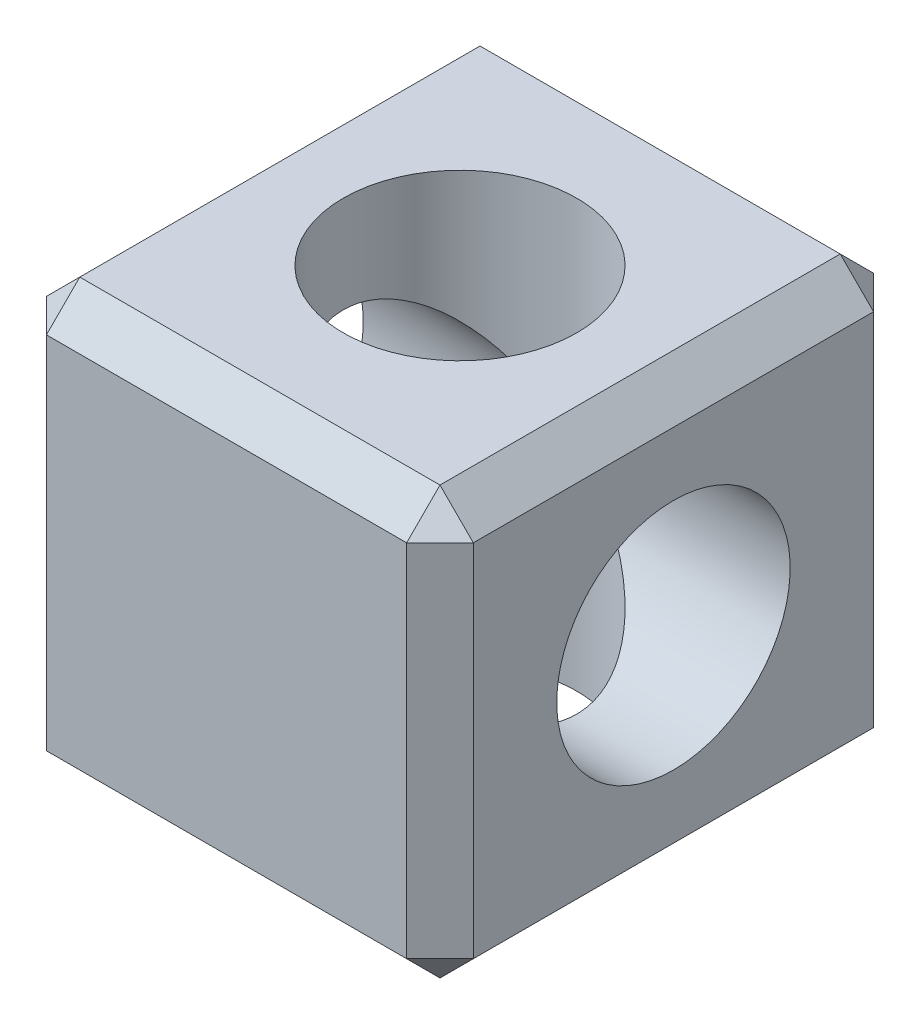
ISO-10303-21;
HEADER;
FILE_DESCRIPTION(('STEP AP214'),'2;1');
FILE_NAME('part.step','',(''),(''),'','','');
FILE_SCHEMA(('AUTOMOTIVE_DESIGN { 1 0 10303 214 1 1 1 1 }'));
ENDSEC;
DATA;
#1=APPLICATION_CONTEXT('core data for automotive mechanical design processes');
#2=APPLICATION_PROTOCOL_DEFINITION('international standard','automotive_design',2000,#1);
#3=PRODUCT_CONTEXT('',#1,'mechanical');
#4=PRODUCT('Part','Part','',(#3));
#5=PRODUCT_RELATED_PRODUCT_CATEGORY('part','',(#4));
#6=PRODUCT_DEFINITION_FORMATION('','',#4);
#7=PRODUCT_DEFINITION_CONTEXT('part definition',#1,'design');
#8=PRODUCT_DEFINITION('design','',#6,#7);
#9=PRODUCT_DEFINITION_SHAPE('','',#8);
#10=(LENGTH_UNIT() NAMED_UNIT(*) SI_UNIT(.MILLI.,.METRE.));
#11=(NAMED_UNIT(*) PLANE_ANGLE_UNIT() SI_UNIT($,.RADIAN.));
#12=(NAMED_UNIT(*) SI_UNIT($,.STERADIAN.) SOLID_ANGLE_UNIT());
#13=UNCERTAINTY_MEASURE_WITH_UNIT(LENGTH_MEASURE(1.E-05),#10,'distance_accuracy_value','');
#14=(GEOMETRIC_REPRESENTATION_CONTEXT(3) GLOBAL_UNCERTAINTY_ASSIGNED_CONTEXT((#13)) GLOBAL_UNIT_ASSIGNED_CONTEXT((#10,
#11,#12)) REPRESENTATION_CONTEXT('',''));
#15=CARTESIAN_POINT('',(0.,0.,0.));
#16=DIRECTION('',(0.,0.,1.));
#17=DIRECTION('',(1.,0.,0.));
#18=AXIS2_PLACEMENT_3D('',#15,#16,#17);
#19=CARTESIAN_POINT('',(0.,-32.,35.));
#20=DIRECTION('',(0.,1.,0.));
#21=DIRECTION('',(-1.,0.,0.));
#22=AXIS2_PLACEMENT_3D('',#19,#20,#21);
#23=CYLINDRICAL_SURFACE('',#22,17.5);
#24=CARTESIAN_POINT('',(0.,32.,35.));
#25=DIRECTION('',(0.,1.,0.));
#26=DIRECTION('',(-1.,0.,0.));
#27=AXIS2_PLACEMENT_3D('',#24,#25,#26);
#28=CIRCLE('',#27,17.5);
#29=CARTESIAN_POINT('',(-17.5,32.,35.));
#30=VERTEX_POINT('',#29);
#31=EDGE_CURVE('E266',#30,#30,#28,.T.);
#32=ORIENTED_EDGE('',*,*,#31,.T.);
#33=EDGE_LOOP('',(#32));
#34=FACE_BOUND('',#33,.T.);
#35=CARTESIAN_POINT('',(0.,0.,35.));
#36=DIRECTION('',(-0.707106781186548,0.707106781186547,0.));
#37=DIRECTION('',(0.707106781186547,0.707106781186548,0.));
#38=AXIS2_PLACEMENT_3D('',#35,#36,#37);
#39=ELLIPSE('',#38,24.7487373415292,17.5);
#40=CARTESIAN_POINT('',(0.,0.,17.5));
#41=VERTEX_POINT('',#40);
#42=CARTESIAN_POINT('',(0.,0.,52.5));
#43=VERTEX_POINT('',#42);
#44=EDGE_CURVE('E145',#41,#43,#39,.F.);
#45=ORIENTED_EDGE('',*,*,#44,.T.);
#46=CARTESIAN_POINT('',(0.,0.,35.));
#47=DIRECTION('',(0.707106781186547,0.707106781186548,0.));
#48=DIRECTION('',(-0.707106781186548,0.707106781186547,0.));
#49=AXIS2_PLACEMENT_3D('',#46,#47,#48);
#50=ELLIPSE('',#49,24.7487373415292,17.5);
#51=EDGE_CURVE('E140',#43,#41,#50,.F.);
#52=ORIENTED_EDGE('',*,*,#51,.T.);
#53=EDGE_LOOP('',(#45,#52));
#54=FACE_BOUND('',#53,.T.);
#55=ADVANCED_FACE('F43',(#34,#54),#23,.F.);
#56=CARTESIAN_POINT('',(-32.,32.,70.));
#57=DIRECTION('',(1.,0.,0.));
#58=DIRECTION('',(0.,0.,-1.));
#59=AXIS2_PLACEMENT_3D('',#56,#57,#58);
#60=PLANE('',#59);
#61=DIRECTION('',(0.,-1.,0.));
#62=VECTOR('',#61,1.);
#63=CARTESIAN_POINT('',(-32.,-32.,4.99999999999999));
#64=LINE('',#63,#62);
#65=CARTESIAN_POINT('',(-32.,27.,4.99999999999999));
#66=VERTEX_POINT('',#65);
#67=CARTESIAN_POINT('',(-32.,-27.,4.99999999999999));
#68=VERTEX_POINT('',#67);
#69=EDGE_CURVE('E167',#66,#68,#64,.T.);
#70=ORIENTED_EDGE('',*,*,#69,.T.);
#71=DIRECTION('',(0.,0.,1.));
#72=VECTOR('',#71,1.);
#73=CARTESIAN_POINT('',(-32.,-27.,70.));
#74=LINE('',#73,#72);
#75=CARTESIAN_POINT('',(-32.,-27.,65.));
#76=VERTEX_POINT('',#75);
#77=EDGE_CURVE('E168',#68,#76,#74,.T.);
#78=ORIENTED_EDGE('',*,*,#77,.T.);
#79=DIRECTION('',(0.,1.,0.));
#80=VECTOR('',#79,1.);
#81=CARTESIAN_POINT('',(-32.,32.,65.));
#82=LINE('',#81,#80);
#83=CARTESIAN_POINT('',(-32.,27.,65.));
#84=VERTEX_POINT('',#83);
#85=EDGE_CURVE('E169',#76,#84,#82,.T.);
#86=ORIENTED_EDGE('',*,*,#85,.T.);
#87=DIRECTION('',(0.,0.,-1.));
#88=VECTOR('',#87,1.);
#89=CARTESIAN_POINT('',(-32.,27.,70.));
#90=LINE('',#89,#88);
#91=EDGE_CURVE('E163',#84,#66,#90,.T.);
#92=ORIENTED_EDGE('',*,*,#91,.T.);
#93=EDGE_LOOP('',(#70,#78,#86,#92));
#94=FACE_BOUND('',#93,.T.);
#95=CARTESIAN_POINT('',(-32.,0.,35.));
#96=DIRECTION('',(1.,0.,0.));
#97=DIRECTION('',(0.,1.,0.));
#98=AXIS2_PLACEMENT_3D('',#95,#96,#97);
#99=CIRCLE('',#98,17.5);
#100=CARTESIAN_POINT('',(-32.,17.5,35.));
#101=VERTEX_POINT('',#100);
#102=EDGE_CURVE('E261',#101,#101,#99,.T.);
#103=ORIENTED_EDGE('',*,*,#102,.T.);
#104=EDGE_LOOP('',(#103));
#105=FACE_BOUND('',#104,.T.);
#106=ADVANCED_FACE('F352',(#94,#105),#60,.F.);
#107=CARTESIAN_POINT('',(32.,-32.,70.));
#108=DIRECTION('',(0.,1.,0.));
#109=DIRECTION('',(-1.,0.,0.));
#110=AXIS2_PLACEMENT_3D('',#107,#108,#109);
#111=PLANE('',#110);
#112=CARTESIAN_POINT('',(0.,-32.,35.));
#113=DIRECTION('',(0.,1.,0.));
#114=DIRECTION('',(-1.,0.,0.));
#115=AXIS2_PLACEMENT_3D('',#112,#113,#114);
#116=CIRCLE('',#115,17.5);
#117=CARTESIAN_POINT('',(-17.5,-32.,35.));
#118=VERTEX_POINT('',#117);
#119=EDGE_CURVE('E267',#118,#118,#116,.T.);
#120=ORIENTED_EDGE('',*,*,#119,.T.);
#121=EDGE_LOOP('',(#120));
#122=FACE_BOUND('',#121,.T.);
#123=DIRECTION('',(-1.,0.,0.));
#124=VECTOR('',#123,1.);
#125=CARTESIAN_POINT('',(32.,-32.,65.));
#126=LINE('',#125,#124);
#127=CARTESIAN_POINT('',(27.,-32.,65.));
#128=VERTEX_POINT('',#127);
#129=CARTESIAN_POINT('',(-27.,-32.,65.));
#130=VERTEX_POINT('',#129);
#131=EDGE_CURVE('E157',#128,#130,#126,.T.);
#132=ORIENTED_EDGE('',*,*,#131,.T.);
#133=DIRECTION('',(0.,0.,-1.));
#134=VECTOR('',#133,1.);
#135=CARTESIAN_POINT('',(-27.,-32.,70.));
#136=LINE('',#135,#134);
#137=CARTESIAN_POINT('',(-27.,-32.,0.));
#138=VERTEX_POINT('',#137);
#139=EDGE_CURVE('E161',#130,#138,#136,.T.);
#140=ORIENTED_EDGE('',*,*,#139,.T.);
#141=DIRECTION('',(1.,0.,0.));
#142=VECTOR('',#141,1.);
#143=CARTESIAN_POINT('',(32.,-32.,0.));
#144=LINE('',#143,#142);
#145=CARTESIAN_POINT('',(27.,-32.,0.));
#146=VERTEX_POINT('',#145);
#147=EDGE_CURVE('E147',#138,#146,#144,.T.);
#148=ORIENTED_EDGE('',*,*,#147,.T.);
#149=DIRECTION('',(0.,0.,1.));
#150=VECTOR('',#149,1.);
#151=CARTESIAN_POINT('',(27.,-32.,70.));
#152=LINE('',#151,#150);
#153=EDGE_CURVE('E155',#146,#128,#152,.T.);
#154=ORIENTED_EDGE('',*,*,#153,.T.);
#155=EDGE_LOOP('',(#132,#140,#148,#154));
#156=FACE_BOUND('',#155,.T.);
#157=ADVANCED_FACE('F279',(#122,#156),#111,.F.);
#158=CARTESIAN_POINT('',(32.,32.,70.));
#159=DIRECTION('',(-1.,0.,0.));
#160=DIRECTION('',(0.,-1.,0.));
#161=AXIS2_PLACEMENT_3D('',#158,#159,#160);
#162=PLANE('',#161);
#163=DIRECTION('',(0.,-1.,0.));
#164=VECTOR('',#163,1.);
#165=CARTESIAN_POINT('',(32.,32.,65.));
#166=LINE('',#165,#164);
#167=CARTESIAN_POINT('',(32.,27.,65.));
#168=VERTEX_POINT('',#167);
#169=CARTESIAN_POINT('',(32.,-27.,65.));
#170=VERTEX_POINT('',#169);
#171=EDGE_CURVE('E188',#168,#170,#166,.T.);
#172=ORIENTED_EDGE('',*,*,#171,.T.);
#173=DIRECTION('',(0.,0.,-1.));
#174=VECTOR('',#173,1.);
#175=CARTESIAN_POINT('',(32.,-27.,70.));
#176=LINE('',#175,#174);
#177=CARTESIAN_POINT('',(32.,-27.,4.99999999999999));
#178=VERTEX_POINT('',#177);
#179=EDGE_CURVE('E186',#170,#178,#176,.T.);
#180=ORIENTED_EDGE('',*,*,#179,.T.);
#181=DIRECTION('',(0.,1.,0.));
#182=VECTOR('',#181,1.);
#183=CARTESIAN_POINT('',(32.,32.,4.99999999999999));
#184=LINE('',#183,#182);
#185=CARTESIAN_POINT('',(32.,27.,4.99999999999999));
#186=VERTEX_POINT('',#185);
#187=EDGE_CURVE('E184',#178,#186,#184,.T.);
#188=ORIENTED_EDGE('',*,*,#187,.T.);
#189=DIRECTION('',(0.,0.,1.));
#190=VECTOR('',#189,1.);
#191=CARTESIAN_POINT('',(32.,27.,70.));
#192=LINE('',#191,#190);
#193=EDGE_CURVE('E185',#186,#168,#192,.T.);
#194=ORIENTED_EDGE('',*,*,#193,.T.);
#195=EDGE_LOOP('',(#172,#180,#188,#194));
#196=FACE_BOUND('',#195,.T.);
#197=CARTESIAN_POINT('',(32.,0.,35.));
#198=DIRECTION('',(1.,0.,0.));
#199=DIRECTION('',(0.,1.,0.));
#200=AXIS2_PLACEMENT_3D('',#197,#198,#199);
#201=CIRCLE('',#200,17.5);
#202=CARTESIAN_POINT('',(32.,17.5,35.));
#203=VERTEX_POINT('',#202);
#204=EDGE_CURVE('E254',#203,#203,#201,.T.);
#205=ORIENTED_EDGE('',*,*,#204,.F.);
#206=EDGE_LOOP('',(#205));
#207=FACE_BOUND('',#206,.T.);
#208=ADVANCED_FACE('F378',(#196,#207),#162,.F.);
#209=CARTESIAN_POINT('',(32.,32.,70.));
#210=DIRECTION('',(0.,-1.,0.));
#211=DIRECTION('',(1.,0.,0.));
#212=AXIS2_PLACEMENT_3D('',#209,#210,#211);
#213=PLANE('',#212);
#214=DIRECTION('',(-1.,0.,0.));
#215=VECTOR('',#214,1.);
#216=CARTESIAN_POINT('',(-32.,32.,4.99999999999999));
#217=LINE('',#216,#215);
#218=CARTESIAN_POINT('',(27.,32.,4.99999999999999));
#219=VERTEX_POINT('',#218);
#220=CARTESIAN_POINT('',(-27.,32.,4.99999999999999));
#221=VERTEX_POINT('',#220);
#222=EDGE_CURVE('E69',#219,#221,#217,.T.);
#223=ORIENTED_EDGE('',*,*,#222,.T.);
#224=DIRECTION('',(0.,0.,1.));
#225=VECTOR('',#224,1.);
#226=CARTESIAN_POINT('',(-27.,32.,70.));
#227=LINE('',#226,#225);
#228=CARTESIAN_POINT('',(-27.,32.,65.));
#229=VERTEX_POINT('',#228);
#230=EDGE_CURVE('E11',#221,#229,#227,.T.);
#231=ORIENTED_EDGE('',*,*,#230,.T.);
#232=DIRECTION('',(1.,0.,0.));
#233=VECTOR('',#232,1.);
#234=CARTESIAN_POINT('',(32.,32.,65.));
#235=LINE('',#234,#233);
#236=CARTESIAN_POINT('',(27.,32.,65.));
#237=VERTEX_POINT('',#236);
#238=EDGE_CURVE('E52',#229,#237,#235,.T.);
#239=ORIENTED_EDGE('',*,*,#238,.T.);
#240=DIRECTION('',(0.,0.,-1.));
#241=VECTOR('',#240,1.);
#242=CARTESIAN_POINT('',(27.,32.,70.));
#243=LINE('',#242,#241);
#244=EDGE_CURVE('E197',#237,#219,#243,.T.);
#245=ORIENTED_EDGE('',*,*,#244,.T.);
#246=EDGE_LOOP('',(#223,#231,#239,#245));
#247=FACE_BOUND('',#246,.T.);
#248=ORIENTED_EDGE('',*,*,#31,.F.);
#249=EDGE_LOOP('',(#248));
#250=FACE_BOUND('',#249,.T.);
#251=ADVANCED_FACE('F322',(#247,#250),#213,.F.);
#252=CARTESIAN_POINT('',(0.,0.,70.));
#253=DIRECTION('',(0.,0.,-1.));
#254=DIRECTION('',(-1.,0.,0.));
#255=AXIS2_PLACEMENT_3D('',#252,#253,#254);
#256=PLANE('',#255);
#257=DIRECTION('',(-1.,0.,0.));
#258=VECTOR('',#257,1.);
#259=CARTESIAN_POINT('',(0.,27.,70.));
#260=LINE('',#259,#258);
#261=CARTESIAN_POINT('',(27.,27.,70.));
#262=VERTEX_POINT('',#261);
#263=CARTESIAN_POINT('',(-27.,27.,70.));
#264=VERTEX_POINT('',#263);
#265=EDGE_CURVE('E171',#262,#264,#260,.T.);
#266=ORIENTED_EDGE('',*,*,#265,.T.);
#267=DIRECTION('',(0.,-1.,0.));
#268=VECTOR('',#267,1.);
#269=CARTESIAN_POINT('',(-27.,0.,70.));
#270=LINE('',#269,#268);
#271=CARTESIAN_POINT('',(-27.,-27.,70.));
#272=VERTEX_POINT('',#271);
#273=EDGE_CURVE('E178',#264,#272,#270,.T.);
#274=ORIENTED_EDGE('',*,*,#273,.T.);
#275=DIRECTION('',(1.,0.,0.));
#276=VECTOR('',#275,1.);
#277=CARTESIAN_POINT('',(0.,-27.,70.));
#278=LINE('',#277,#276);
#279=CARTESIAN_POINT('',(27.,-27.,70.));
#280=VERTEX_POINT('',#279);
#281=EDGE_CURVE('E177',#272,#280,#278,.T.);
#282=ORIENTED_EDGE('',*,*,#281,.T.);
#283=DIRECTION('',(0.,1.,0.));
#284=VECTOR('',#283,1.);
#285=CARTESIAN_POINT('',(27.,0.,70.));
#286=LINE('',#285,#284);
#287=EDGE_CURVE('E172',#280,#262,#286,.T.);
#288=ORIENTED_EDGE('',*,*,#287,.T.);
#289=EDGE_LOOP('',(#266,#274,#282,#288));
#290=FACE_BOUND('',#289,.T.);
#291=ADVANCED_FACE('F338',(#290),#256,.F.);
#292=CARTESIAN_POINT('',(0.,0.,0.));
#293=DIRECTION('',(0.,0.,-1.));
#294=DIRECTION('',(-1.,0.,0.));
#295=AXIS2_PLACEMENT_3D('',#292,#293,#294);
#296=PLANE('',#295);
#297=ORIENTED_EDGE('',*,*,#147,.F.);
#298=DIRECTION('',(0.,1.,0.));
#299=VECTOR('',#298,1.);
#300=CARTESIAN_POINT('',(-27.,32.,0.));
#301=LINE('',#300,#299);
#302=CARTESIAN_POINT('',(-27.,27.,0.));
#303=VERTEX_POINT('',#302);
#304=EDGE_CURVE('E195',#138,#303,#301,.T.);
#305=ORIENTED_EDGE('',*,*,#304,.T.);
#306=DIRECTION('',(1.,0.,0.));
#307=VECTOR('',#306,1.);
#308=CARTESIAN_POINT('',(32.,27.,0.));
#309=LINE('',#308,#307);
#310=CARTESIAN_POINT('',(27.,27.,0.));
#311=VERTEX_POINT('',#310);
#312=EDGE_CURVE('E191',#303,#311,#309,.T.);
#313=ORIENTED_EDGE('',*,*,#312,.T.);
#314=DIRECTION('',(0.,-1.,0.));
#315=VECTOR('',#314,1.);
#316=CARTESIAN_POINT('',(27.,-32.,0.));
#317=LINE('',#316,#315);
#318=EDGE_CURVE('E194',#311,#146,#317,.T.);
#319=ORIENTED_EDGE('',*,*,#318,.T.);
#320=EDGE_LOOP('',(#297,#305,#313,#319));
#321=FACE_BOUND('',#320,.T.);
#322=ADVANCED_FACE('F312',(#321),#296,.T.);
#323=CARTESIAN_POINT('',(0.,0.,35.));
#324=DIRECTION('',(-0.707106781186548,0.707106781186547,0.));
#325=DIRECTION('',(0.707106781186547,0.707106781186548,0.));
#326=AXIS2_PLACEMENT_3D('',#323,#324,#325);
#327=ELLIPSE('',#326,24.7487373415292,17.5);
#328=EDGE_CURVE('E136',#41,#43,#327,.T.);
#329=ORIENTED_EDGE('',*,*,#328,.T.);
#330=CARTESIAN_POINT('',(0.,0.,35.));
#331=DIRECTION('',(0.707106781186547,0.707106781186548,0.));
#332=DIRECTION('',(-0.707106781186548,0.707106781186547,0.));
#333=AXIS2_PLACEMENT_3D('',#330,#331,#332);
#334=ELLIPSE('',#333,24.7487373415292,17.5);
#335=EDGE_CURVE('E141',#43,#41,#334,.T.);
#336=ORIENTED_EDGE('',*,*,#335,.T.);
#337=EDGE_LOOP('',(#329,#336));
#338=FACE_BOUND('',#337,.T.);
#339=ORIENTED_EDGE('',*,*,#119,.F.);
#340=EDGE_LOOP('',(#339));
#341=FACE_BOUND('',#340,.T.);
#342=ADVANCED_FACE('F152',(#338,#341),#23,.F.);
#343=CARTESIAN_POINT('',(-32.,0.,35.));
#344=DIRECTION('',(1.,0.,0.));
#345=DIRECTION('',(0.,1.,0.));
#346=AXIS2_PLACEMENT_3D('',#343,#344,#345);
#347=CYLINDRICAL_SURFACE('',#346,17.5);
#348=ORIENTED_EDGE('',*,*,#204,.T.);
#349=EDGE_LOOP('',(#348));
#350=FACE_BOUND('',#349,.T.);
#351=ORIENTED_EDGE('',*,*,#44,.F.);
#352=ORIENTED_EDGE('',*,*,#335,.F.);
#353=EDGE_LOOP('',(#351,#352));
#354=FACE_BOUND('',#353,.T.);
#355=ADVANCED_FACE('F146',(#350,#354),#347,.F.);
#356=ORIENTED_EDGE('',*,*,#102,.F.);
#357=EDGE_LOOP('',(#356));
#358=FACE_BOUND('',#357,.T.);
#359=ORIENTED_EDGE('',*,*,#328,.F.);
#360=ORIENTED_EDGE('',*,*,#51,.F.);
#361=EDGE_LOOP('',(#359,#360));
#362=FACE_BOUND('',#361,.T.);
#363=ADVANCED_FACE('F139',(#358,#362),#347,.F.);
#364=CARTESIAN_POINT('',(27.,27.,70.));
#365=DIRECTION('',(0.577350269189626,0.577350269189626,0.577350269189626));
#366=DIRECTION('',(0.707106781186547,0.,-0.707106781186547));
#367=AXIS2_PLACEMENT_3D('',#364,#365,#366);
#368=PLANE('',#367);
#369=DIRECTION('',(-0.707106781186547,0.,0.707106781186547));
#370=VECTOR('',#369,1.);
#371=CARTESIAN_POINT('',(27.,27.,70.));
#372=LINE('',#371,#370);
#373=EDGE_CURVE('E242',#168,#262,#372,.T.);
#374=ORIENTED_EDGE('',*,*,#373,.F.);
#375=DIRECTION('',(0.707106781186547,-0.707106781186547,0.));
#376=VECTOR('',#375,1.);
#377=CARTESIAN_POINT('',(29.5,29.5,65.));
#378=LINE('',#377,#376);
#379=EDGE_CURVE('E48',#237,#168,#378,.T.);
#380=ORIENTED_EDGE('',*,*,#379,.F.);
#381=DIRECTION('',(0.,0.707106781186548,-0.707106781186548));
#382=VECTOR('',#381,1.);
#383=CARTESIAN_POINT('',(27.,27.,70.));
#384=LINE('',#383,#382);
#385=EDGE_CURVE('E247',#262,#237,#384,.T.);
#386=ORIENTED_EDGE('',*,*,#385,.F.);
#387=EDGE_LOOP('',(#374,#380,#386));
#388=FACE_BOUND('',#387,.T.);
#389=ADVANCED_FACE('F46',(#388),#368,.T.);
#390=CARTESIAN_POINT('',(32.,32.,4.99999999999999));
#391=DIRECTION('',(0.707106781186547,0.,-0.707106781186547));
#392=DIRECTION('',(0.,-1.,0.));
#393=AXIS2_PLACEMENT_3D('',#390,#391,#392);
#394=PLANE('',#393);
#395=DIRECTION('',(-0.707106781186547,0.,-0.707106781186547));
#396=VECTOR('',#395,1.);
#397=CARTESIAN_POINT('',(32.,27.,4.99999999999999));
#398=LINE('',#397,#396);
#399=EDGE_CURVE('E238',#186,#311,#398,.T.);
#400=ORIENTED_EDGE('',*,*,#399,.F.);
#401=ORIENTED_EDGE('',*,*,#187,.F.);
#402=DIRECTION('',(0.577350269189626,0.577350269189626,0.577350269189626));
#403=VECTOR('',#402,1.);
#404=CARTESIAN_POINT('',(51.6666666666667,-7.33333333333334,24.6666666666667));
#405=LINE('',#404,#403);
#406=EDGE_CURVE('E241',#146,#178,#405,.T.);
#407=ORIENTED_EDGE('',*,*,#406,.F.);
#408=ORIENTED_EDGE('',*,*,#318,.F.);
#409=EDGE_LOOP('',(#400,#401,#407,#408));
#410=FACE_BOUND('',#409,.T.);
#411=ADVANCED_FACE('F287',(#410),#394,.T.);
#412=CARTESIAN_POINT('',(27.,32.,70.));
#413=DIRECTION('',(-0.707106781186547,-0.707106781186547,0.));
#414=DIRECTION('',(0.,0.,-1.));
#415=AXIS2_PLACEMENT_3D('',#412,#413,#414);
#416=PLANE('',#415);
#417=ORIENTED_EDGE('',*,*,#379,.T.);
#418=ORIENTED_EDGE('',*,*,#193,.F.);
#419=DIRECTION('',(-0.707106781186547,0.707106781186547,0.));
#420=VECTOR('',#419,1.);
#421=CARTESIAN_POINT('',(32.,27.,4.99999999999999));
#422=LINE('',#421,#420);
#423=EDGE_CURVE('E240',#219,#186,#422,.F.);
#424=ORIENTED_EDGE('',*,*,#423,.F.);
#425=ORIENTED_EDGE('',*,*,#244,.F.);
#426=EDGE_LOOP('',(#417,#418,#424,#425));
#427=FACE_BOUND('',#426,.T.);
#428=ADVANCED_FACE('F342',(#427),#416,.F.);
#429=CARTESIAN_POINT('',(0.,27.,70.));
#430=DIRECTION('',(0.,-0.707106781186547,-0.707106781186547));
#431=DIRECTION('',(-1.,0.,0.));
#432=AXIS2_PLACEMENT_3D('',#429,#430,#431);
#433=PLANE('',#432);
#434=ORIENTED_EDGE('',*,*,#385,.T.);
#435=ORIENTED_EDGE('',*,*,#238,.F.);
#436=DIRECTION('',(0.,-0.707106781186547,0.707106781186547));
#437=VECTOR('',#436,1.);
#438=CARTESIAN_POINT('',(-27.,29.5,67.5));
#439=LINE('',#438,#437);
#440=EDGE_CURVE('E235',#264,#229,#439,.F.);
#441=ORIENTED_EDGE('',*,*,#440,.F.);
#442=ORIENTED_EDGE('',*,*,#265,.F.);
#443=EDGE_LOOP('',(#434,#435,#441,#442));
#444=FACE_BOUND('',#443,.T.);
#445=ADVANCED_FACE('F327',(#444),#433,.F.);
#446=CARTESIAN_POINT('',(27.,0.,70.));
#447=DIRECTION('',(-0.707106781186547,0.,-0.707106781186547));
#448=DIRECTION('',(0.,1.,0.));
#449=AXIS2_PLACEMENT_3D('',#446,#447,#448);
#450=PLANE('',#449);
#451=ORIENTED_EDGE('',*,*,#373,.T.);
#452=ORIENTED_EDGE('',*,*,#287,.F.);
#453=DIRECTION('',(0.707106781186548,0.,-0.707106781186548));
#454=VECTOR('',#453,1.);
#455=CARTESIAN_POINT('',(27.,-27.,70.));
#456=LINE('',#455,#454);
#457=EDGE_CURVE('E232',#170,#280,#456,.F.);
#458=ORIENTED_EDGE('',*,*,#457,.F.);
#459=ORIENTED_EDGE('',*,*,#171,.F.);
#460=EDGE_LOOP('',(#451,#452,#458,#459));
#461=FACE_BOUND('',#460,.T.);
#462=ADVANCED_FACE('F337',(#461),#450,.F.);
#463=CARTESIAN_POINT('',(32.,-27.,70.));
#464=DIRECTION('',(-0.707106781186547,0.707106781186547,0.));
#465=DIRECTION('',(0.,0.,-1.));
#466=AXIS2_PLACEMENT_3D('',#463,#464,#465);
#467=PLANE('',#466);
#468=ORIENTED_EDGE('',*,*,#406,.T.);
#469=ORIENTED_EDGE('',*,*,#179,.F.);
#470=DIRECTION('',(-0.707106781186547,-0.707106781186547,0.));
#471=VECTOR('',#470,1.);
#472=CARTESIAN_POINT('',(29.5,-29.5,65.));
#473=LINE('',#472,#471);
#474=EDGE_CURVE('E229',#128,#170,#473,.F.);
#475=ORIENTED_EDGE('',*,*,#474,.F.);
#476=ORIENTED_EDGE('',*,*,#153,.F.);
#477=EDGE_LOOP('',(#468,#469,#475,#476));
#478=FACE_BOUND('',#477,.T.);
#479=ADVANCED_FACE('F290',(#478),#467,.F.);
#480=CARTESIAN_POINT('',(32.,27.,4.99999999999999));
#481=DIRECTION('',(0.577350269189626,0.577350269189626,-0.577350269189626));
#482=DIRECTION('',(-0.707106781186547,0.,-0.707106781186547));
#483=AXIS2_PLACEMENT_3D('',#480,#481,#482);
#484=PLANE('',#483);
#485=ORIENTED_EDGE('',*,*,#423,.T.);
#486=ORIENTED_EDGE('',*,*,#399,.T.);
#487=DIRECTION('',(0.,0.707106781186548,0.707106781186548));
#488=VECTOR('',#487,1.);
#489=CARTESIAN_POINT('',(27.,29.5,2.5));
#490=LINE('',#489,#488);
#491=EDGE_CURVE('E228',#219,#311,#490,.F.);
#492=ORIENTED_EDGE('',*,*,#491,.F.);
#493=EDGE_LOOP('',(#485,#486,#492));
#494=FACE_BOUND('',#493,.T.);
#495=ADVANCED_FACE('F343',(#494),#484,.T.);
#496=CARTESIAN_POINT('',(-32.,27.,65.));
#497=DIRECTION('',(-0.577350269189626,0.577350269189626,0.577350269189626));
#498=DIRECTION('',(0.707106781186547,0.,0.707106781186547));
#499=AXIS2_PLACEMENT_3D('',#496,#497,#498);
#500=PLANE('',#499);
#501=DIRECTION('',(-0.707106781186547,0.,-0.707106781186547));
#502=VECTOR('',#501,1.);
#503=CARTESIAN_POINT('',(-32.,27.,65.));
#504=LINE('',#503,#502);
#505=EDGE_CURVE('E225',#264,#84,#504,.T.);
#506=ORIENTED_EDGE('',*,*,#505,.F.);
#507=ORIENTED_EDGE('',*,*,#440,.T.);
#508=DIRECTION('',(0.707106781186547,0.707106781186547,0.));
#509=VECTOR('',#508,1.);
#510=CARTESIAN_POINT('',(-32.,27.,65.));
#511=LINE('',#510,#509);
#512=EDGE_CURVE('E63',#84,#229,#511,.T.);
#513=ORIENTED_EDGE('',*,*,#512,.F.);
#514=EDGE_LOOP('',(#506,#507,#513));
#515=FACE_BOUND('',#514,.T.);
#516=ADVANCED_FACE('F335',(#515),#500,.T.);
#517=CARTESIAN_POINT('',(27.,-27.,70.));
#518=DIRECTION('',(0.577350269189626,-0.577350269189626,0.577350269189626));
#519=DIRECTION('',(0.707106781186547,0.,-0.707106781186547));
#520=AXIS2_PLACEMENT_3D('',#517,#518,#519);
#521=PLANE('',#520);
#522=ORIENTED_EDGE('',*,*,#474,.T.);
#523=ORIENTED_EDGE('',*,*,#457,.T.);
#524=DIRECTION('',(0.,0.707106781186547,0.707106781186547));
#525=VECTOR('',#524,1.);
#526=CARTESIAN_POINT('',(27.,-27.,70.));
#527=LINE('',#526,#525);
#528=EDGE_CURVE('E218',#128,#280,#527,.T.);
#529=ORIENTED_EDGE('',*,*,#528,.F.);
#530=EDGE_LOOP('',(#522,#523,#529));
#531=FACE_BOUND('',#530,.T.);
#532=ADVANCED_FACE('F293',(#531),#521,.T.);
#533=CARTESIAN_POINT('',(32.,32.,4.99999999999999));
#534=DIRECTION('',(0.,0.707106781186547,-0.707106781186547));
#535=DIRECTION('',(1.,0.,0.));
#536=AXIS2_PLACEMENT_3D('',#533,#534,#535);
#537=PLANE('',#536);
#538=ORIENTED_EDGE('',*,*,#491,.T.);
#539=ORIENTED_EDGE('',*,*,#312,.F.);
#540=DIRECTION('',(0.,-0.707106781186547,-0.707106781186547));
#541=VECTOR('',#540,1.);
#542=CARTESIAN_POINT('',(-27.,27.,0.));
#543=LINE('',#542,#541);
#544=EDGE_CURVE('E216',#221,#303,#543,.T.);
#545=ORIENTED_EDGE('',*,*,#544,.F.);
#546=ORIENTED_EDGE('',*,*,#222,.F.);
#547=EDGE_LOOP('',(#538,#539,#545,#546));
#548=FACE_BOUND('',#547,.T.);
#549=ADVANCED_FACE('F318',(#548),#537,.T.);
#550=CARTESIAN_POINT('',(-32.,27.,70.));
#551=DIRECTION('',(0.707106781186547,-0.707106781186547,0.));
#552=DIRECTION('',(0.,0.,-1.));
#553=AXIS2_PLACEMENT_3D('',#550,#551,#552);
#554=PLANE('',#553);
#555=ORIENTED_EDGE('',*,*,#512,.T.);
#556=ORIENTED_EDGE('',*,*,#230,.F.);
#557=DIRECTION('',(-0.707106781186547,-0.707106781186547,0.));
#558=VECTOR('',#557,1.);
#559=CARTESIAN_POINT('',(-29.5,29.5,4.99999999999999));
#560=LINE('',#559,#558);
#561=EDGE_CURVE('E213',#66,#221,#560,.F.);
#562=ORIENTED_EDGE('',*,*,#561,.F.);
#563=ORIENTED_EDGE('',*,*,#91,.F.);
#564=EDGE_LOOP('',(#555,#556,#562,#563));
#565=FACE_BOUND('',#564,.T.);
#566=ADVANCED_FACE('F323',(#565),#554,.F.);
#567=CARTESIAN_POINT('',(-27.,0.,70.));
#568=DIRECTION('',(0.707106781186547,0.,-0.707106781186547));
#569=DIRECTION('',(0.,-1.,0.));
#570=AXIS2_PLACEMENT_3D('',#567,#568,#569);
#571=PLANE('',#570);
#572=ORIENTED_EDGE('',*,*,#505,.T.);
#573=ORIENTED_EDGE('',*,*,#85,.F.);
#574=DIRECTION('',(0.707106781186547,0.,0.707106781186547));
#575=VECTOR('',#574,1.);
#576=CARTESIAN_POINT('',(-32.,-27.,65.));
#577=LINE('',#576,#575);
#578=EDGE_CURVE('E209',#272,#76,#577,.F.);
#579=ORIENTED_EDGE('',*,*,#578,.F.);
#580=ORIENTED_EDGE('',*,*,#273,.F.);
#581=EDGE_LOOP('',(#572,#573,#579,#580));
#582=FACE_BOUND('',#581,.T.);
#583=ADVANCED_FACE('F331',(#582),#571,.F.);
#584=CARTESIAN_POINT('',(0.,-27.,70.));
#585=DIRECTION('',(0.,0.707106781186547,-0.707106781186547));
#586=DIRECTION('',(1.,0.,0.));
#587=AXIS2_PLACEMENT_3D('',#584,#585,#586);
#588=PLANE('',#587);
#589=ORIENTED_EDGE('',*,*,#528,.T.);
#590=ORIENTED_EDGE('',*,*,#281,.F.);
#591=DIRECTION('',(0.,-0.707106781186548,-0.707106781186548));
#592=VECTOR('',#591,1.);
#593=CARTESIAN_POINT('',(-27.,-29.5,67.5));
#594=LINE('',#593,#592);
#595=EDGE_CURVE('E208',#130,#272,#594,.F.);
#596=ORIENTED_EDGE('',*,*,#595,.F.);
#597=ORIENTED_EDGE('',*,*,#131,.F.);
#598=EDGE_LOOP('',(#589,#590,#596,#597));
#599=FACE_BOUND('',#598,.T.);
#600=ADVANCED_FACE('F299',(#599),#588,.F.);
#601=CARTESIAN_POINT('',(-27.,27.,0.));
#602=DIRECTION('',(-0.577350269189626,0.577350269189626,-0.577350269189626));
#603=DIRECTION('',(-0.707106781186547,0.,0.707106781186547));
#604=AXIS2_PLACEMENT_3D('',#601,#602,#603);
#605=PLANE('',#604);
#606=ORIENTED_EDGE('',*,*,#561,.T.);
#607=ORIENTED_EDGE('',*,*,#544,.T.);
#608=DIRECTION('',(-0.707106781186547,0.,0.707106781186547));
#609=VECTOR('',#608,1.);
#610=CARTESIAN_POINT('',(-27.,27.,0.));
#611=LINE('',#610,#609);
#612=EDGE_CURVE('E202',#66,#303,#611,.F.);
#613=ORIENTED_EDGE('',*,*,#612,.F.);
#614=EDGE_LOOP('',(#606,#607,#613));
#615=FACE_BOUND('',#614,.T.);
#616=ADVANCED_FACE('F321',(#615),#605,.T.);
#617=CARTESIAN_POINT('',(-32.,-27.,65.));
#618=DIRECTION('',(-0.577350269189626,-0.577350269189626,0.577350269189626));
#619=DIRECTION('',(0.707106781186547,0.,0.707106781186547));
#620=AXIS2_PLACEMENT_3D('',#617,#618,#619);
#621=PLANE('',#620);
#622=ORIENTED_EDGE('',*,*,#595,.T.);
#623=ORIENTED_EDGE('',*,*,#578,.T.);
#624=DIRECTION('',(-0.707106781186547,0.707106781186547,0.));
#625=VECTOR('',#624,1.);
#626=CARTESIAN_POINT('',(-32.,-27.,65.));
#627=LINE('',#626,#625);
#628=EDGE_CURVE('E201',#130,#76,#627,.T.);
#629=ORIENTED_EDGE('',*,*,#628,.F.);
#630=EDGE_LOOP('',(#622,#623,#629));
#631=FACE_BOUND('',#630,.T.);
#632=ADVANCED_FACE('F304',(#631),#621,.T.);
#633=CARTESIAN_POINT('',(-32.,32.,4.99999999999999));
#634=DIRECTION('',(-0.707106781186547,0.,-0.707106781186547));
#635=DIRECTION('',(0.,1.,0.));
#636=AXIS2_PLACEMENT_3D('',#633,#634,#635);
#637=PLANE('',#636);
#638=ORIENTED_EDGE('',*,*,#612,.T.);
#639=ORIENTED_EDGE('',*,*,#304,.F.);
#640=DIRECTION('',(0.577350269189626,-0.577350269189626,-0.577350269189626));
#641=VECTOR('',#640,1.);
#642=CARTESIAN_POINT('',(-51.6666666666667,-7.33333333333334,24.6666666666667));
#643=LINE('',#642,#641);
#644=EDGE_CURVE('E203',#68,#138,#643,.T.);
#645=ORIENTED_EDGE('',*,*,#644,.F.);
#646=ORIENTED_EDGE('',*,*,#69,.F.);
#647=EDGE_LOOP('',(#638,#639,#645,#646));
#648=FACE_BOUND('',#647,.T.);
#649=ADVANCED_FACE('F315',(#648),#637,.T.);
#650=CARTESIAN_POINT('',(-27.,-32.,70.));
#651=DIRECTION('',(0.707106781186547,0.707106781186547,0.));
#652=DIRECTION('',(0.,0.,-1.));
#653=AXIS2_PLACEMENT_3D('',#650,#651,#652);
#654=PLANE('',#653);
#655=ORIENTED_EDGE('',*,*,#628,.T.);
#656=ORIENTED_EDGE('',*,*,#77,.F.);
#657=ORIENTED_EDGE('',*,*,#644,.T.);
#658=ORIENTED_EDGE('',*,*,#139,.F.);
#659=EDGE_LOOP('',(#655,#656,#657,#658));
#660=FACE_BOUND('',#659,.T.);
#661=ADVANCED_FACE('F307',(#660),#654,.F.);
#662=CLOSED_SHELL('',(#55,#106,#157,#208,#251,#291,#322,#342,#355,#363,#389,#411,#428,#445,#462,
#479,#495,#516,#532,#549,#566,#583,#600,#616,#632,#649,#661));
#663=MANIFOLD_SOLID_BREP('B2',#662);
#664=ADVANCED_BREP_SHAPE_REPRESENTATION('',(#18,#663),#14);
#665=SHAPE_DEFINITION_REPRESENTATION(#9,#664);
ENDSEC;
END-ISO-10303-21;
